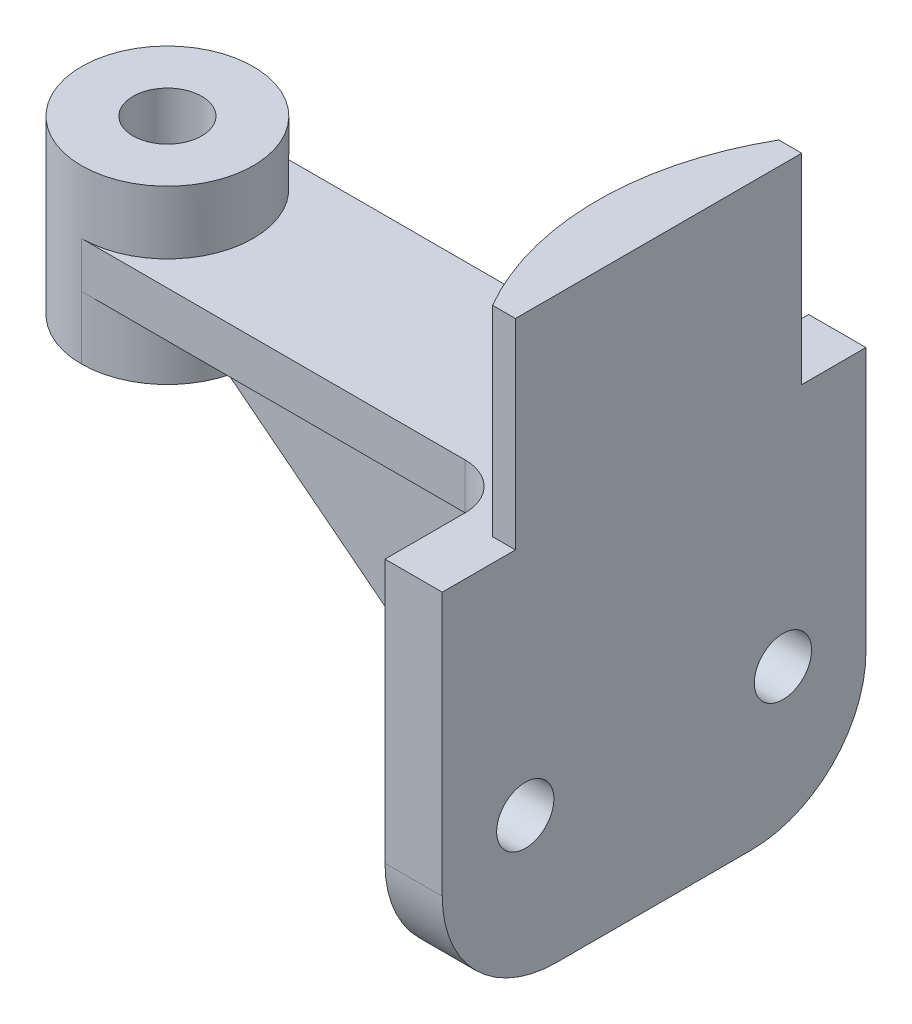
SolidWorks part; units mm, degrees
material "Plain Carbon Steel"
ref_plane "Front Plane" through (0, 0, 0) normal (0, 0, 1) x (1, 0, 0)
ref_plane "Top Plane" through (0, 0, 0) normal (0, 1, 0) x (1, 0, 0)
ref_plane "Right Plane" through (0, 0, 0) normal (1, 0, 0) x (0, 0, -1)
sketch "Hub Profile" plane through (0, 0, 0) normal (0, 1, 0) x (1, 0, 0)
  circle A0 centre (0, 0) radius 15
  dimension "D1" = 30
extrude "Hub Ø30" add sketch "Hub Profile" along normal blind 30
sketch "Bore Profile" plane through (0, 30, 0) normal (0, 1, 0) x (1, 0, 0)
  circle A0 centre (0, 0) radius 6
  dimension "D1" = 12
extrude "Bore Ø12" cut sketch "Bore Profile" against normal blind 60
ref_plane "Arm Plane" through (0, 15, 0) normal (0, 1, 0) x (1, 0, 0)
sketch "Arm Profile" plane through (0, 15, 0) normal (0, 1, 0) x (1, 0, 0)
  line L1 (85, 0) -> (85, 37)
  line L2 (85, 37) -> (75, 37)
  line L3 (75, 37) -> (75, 23)
  line L4 (67, 15) -> (0, 15)
  line L5 (0, -15) -> (67, -15)
  line L6 (85, 0) -> (85, -37)
  line L7 (85, -37) -> (75, -37)
  line L8 (75, -37) -> (75, -23)
  circle A0 centre (0, 0) radius 15 construction
  arc A1 (75, 23) -> (67, 15) centre (67, 23) cw
  arc A2 (75, -23) -> (67, -15) centre (67, -23) ccw
  arc A3 (0, -15) -> (0, 15) centre (0, 0) ccw
  dimension "D1" = 8
  dimension "D2" = 8
  dimension "D3" = 74
  dimension "D4" = 67
  dimension "D5" = 30
  dimension "D6" = 67
  dimension "D7" = 10
  dimension "D8" = 37
  dimension "D9" = 37
extrude "Arm" add sketch "Arm Profile" along normal mid plane 8
sketch "Mounting Plate Profile" plane through (0, 19, 0) normal (0, 1, 0) x (1, 0, 0)
  line L0 (85, 0.7809) -> (85, 25.7809)
  line L1 (85, -37) -> (85, 37) construction
  line L2 (85, 25.7809) -> (81, 25.7809)
  line L3 (85, 0.7809) -> (85, -24.2191)
  line L4 (85, -24.2191) -> (81, -24.2191)
  arc A0 (81, -24.2191) -> (81, 25.7809) centre (124.3013, 0.7809) cw
  dimension "D6" = 50
  dimension "D1" = 25
  dimension "D2" = 4
  dimension "D3" = 25.7809
  dimension "D4" = 25
  dimension "D5" = 4
extrude "Mounting Plate" add sketch "Mounting Plate Profile" along normal blind 35
sketch "Plate Lug Profile" plane through (85, 0, 0) normal (1, 0, 0) x (0, 0, -1)
  line L0 (-37, 11) -> (-37, -27)
  line L1 (-17, -47) -> (17, -47)
  line L2 (37, -27) -> (37, 11)
  line L3 (-37, 11) -> (37, 11)
  arc A0 (17, -47) -> (37, -27) centre (17, -27) ccw
  arc A1 (-37, -27) -> (-17, -47) centre (-17, -27) ccw
  dimension "D1" = 20
  dimension "D2" = 27
extrude "Plate Lug" add sketch "Plate Lug Profile" against normal blind 10
sketch "Mounting Holes Profile" plane through (85, 0, 0) normal (1, 0, 0) x (0, 0, -1)
  line L0 (-24.2191, 54) -> (25.7809, 54) construction
  line L4 (37, 19) -> (37, -27) construction
  line L5 (-37, 19) -> (-24.2191, 19) construction
  circle A0 centre (22.5, -22) radius 5
  circle A1 centre (-22.5, -22) radius 5
  dimension "D1" = 10
  dimension "D2" = 10
  dimension "D3" = 76
  dimension "D4" = 59.5
  dimension "D5" = 41
  dimension "D6" = 14.5
extrude "Mounting Holes 2xØ10" cut sketch "Mounting Holes Profile" against normal blind 87
sketch "Rib Line" plane through (0, 0, 0) normal (0, 0, 1) x (1, 0, 0)
  line L0 (15, 0) -> (75, -47)
rib "Support Rib" sketch "Rib Line" sketch "Rib Line" thickness 8 extrusion direction parallel to sketch draft on no parameters "D1"=8
